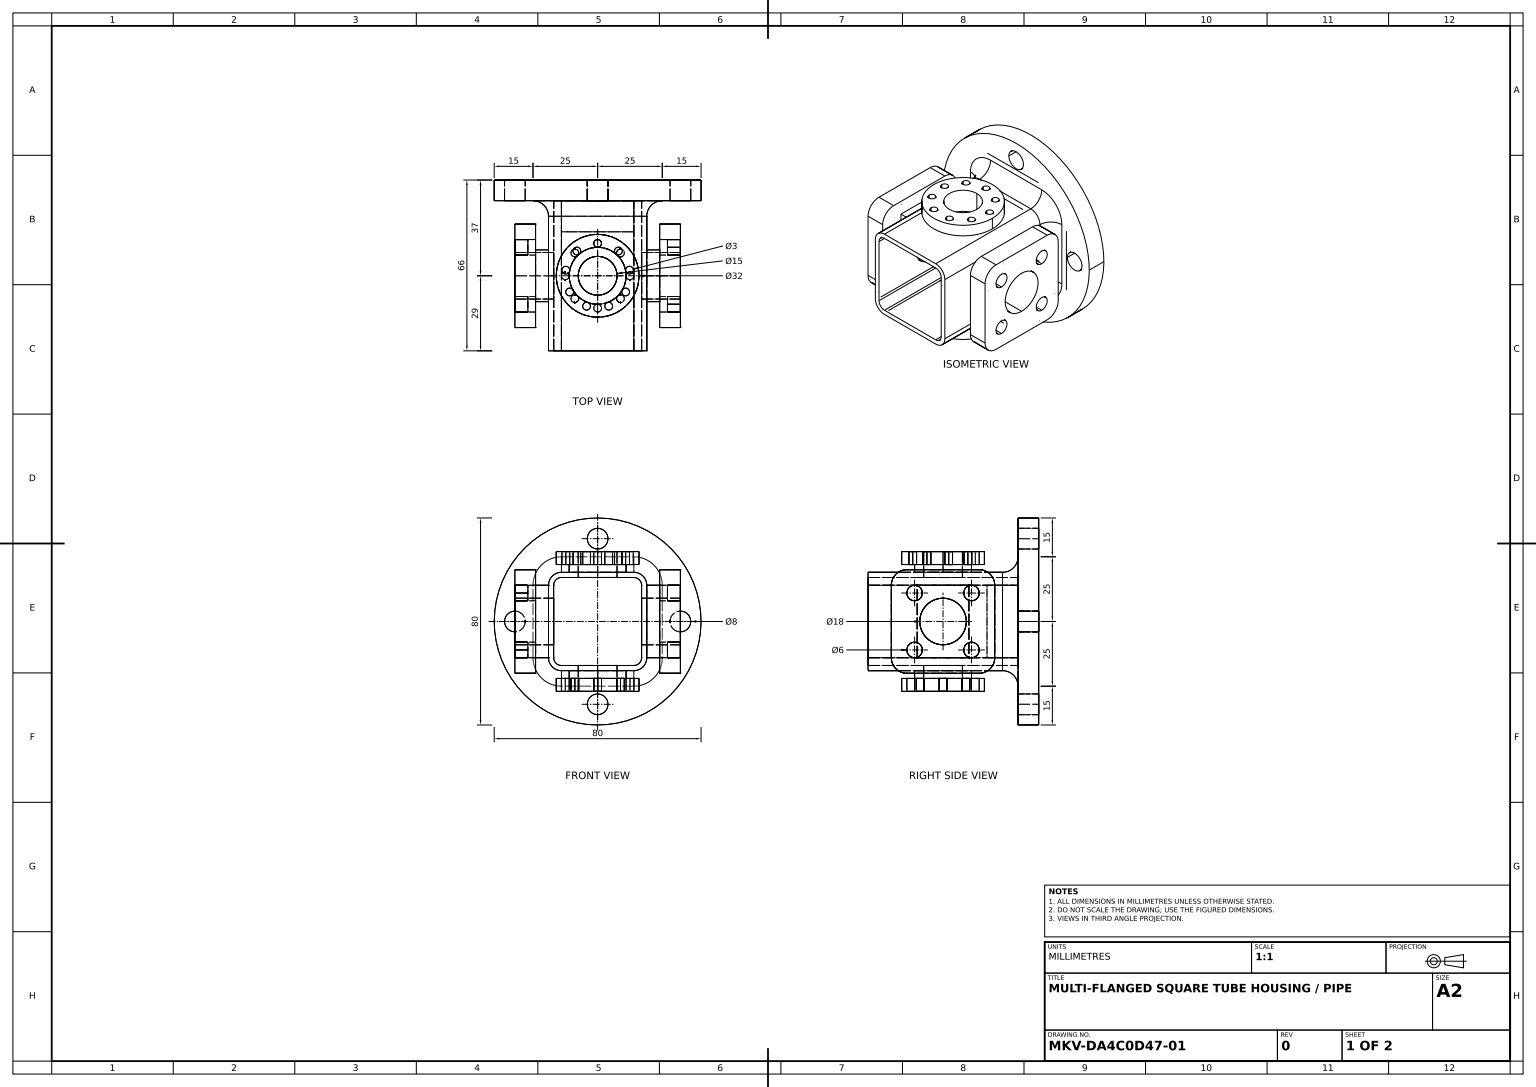
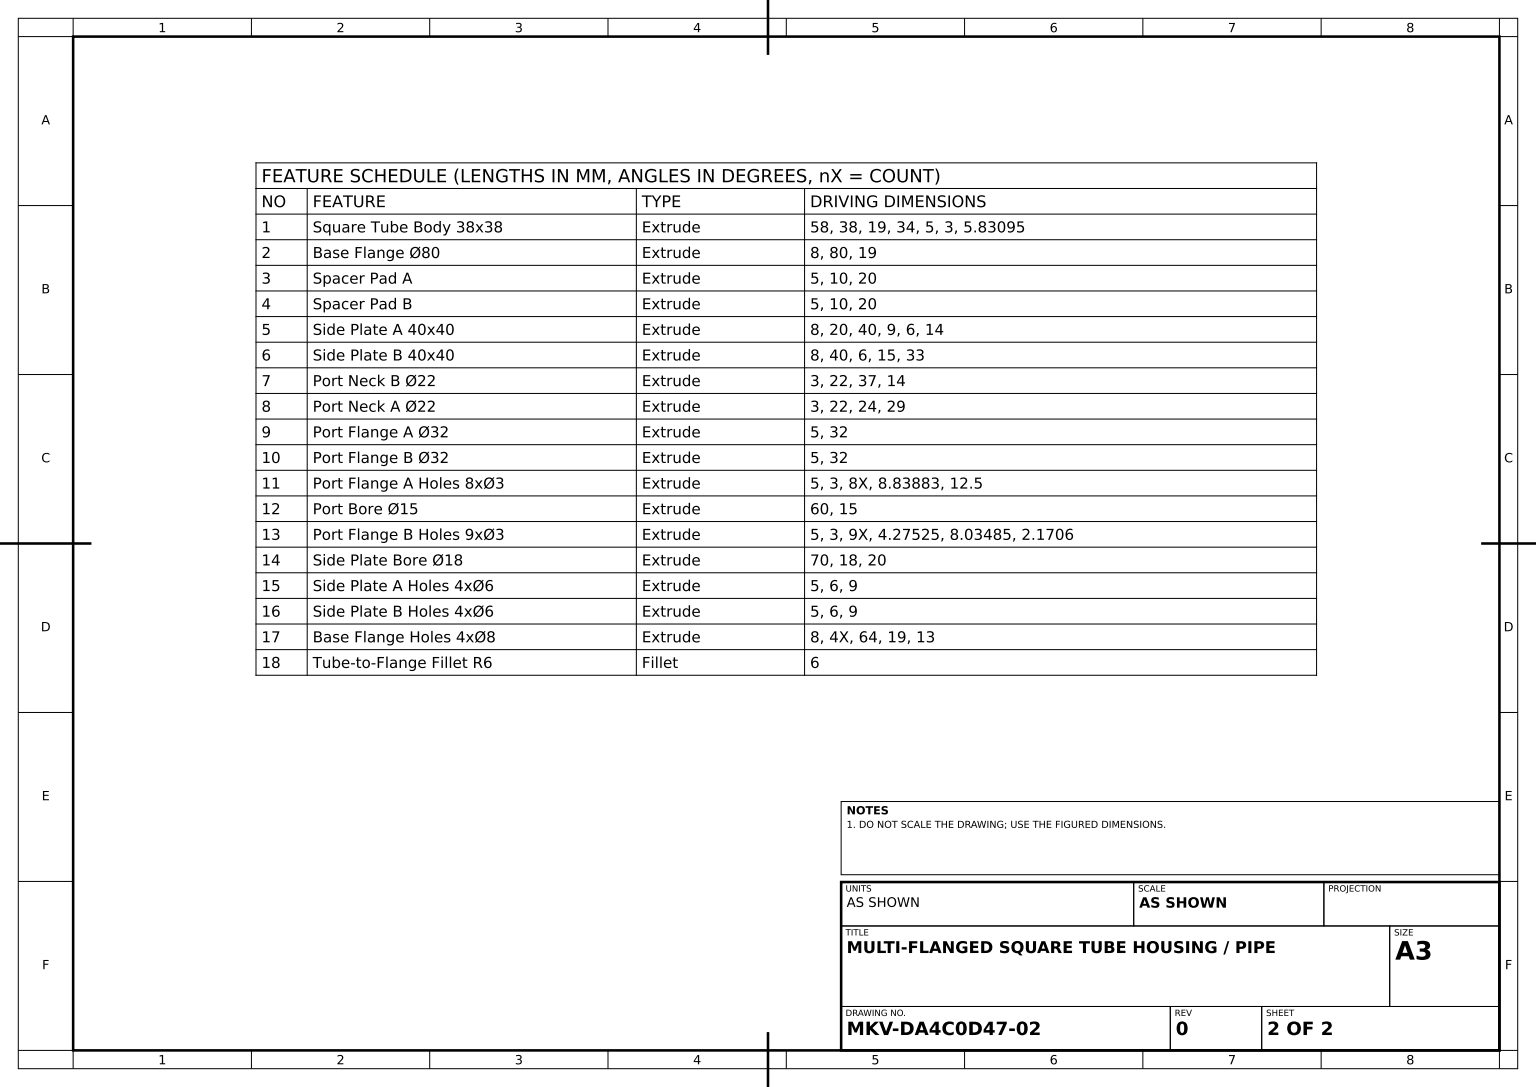
SolidWorks part; units mm, degrees
material "Plain Carbon Steel"
ref_plane "Front Plane" through (0, 0, 0) normal (0, 0, 1) x (1, 0, 0)
ref_plane "Top Plane" through (0, 0, 0) normal (0, 1, 0) x (1, 0, 0)
ref_plane "Right Plane" through (0, 0, 0) normal (1, 0, 0) x (0, 0, -1)
sketch "Square Tube Profile Sketch" plane through (0, 0, 0) normal (0, 0, 1) x (1, 0, 0)
  line L0 (5, 0) -> (33, 0)
  line L1 (38, -5) -> (38, -33)
  line L2 (33, -38) -> (5, -38)
  line L3 (0, -33) -> (0, -5)
  line L4 (5, -2) -> (33, -2)
  line L9 (36, -5) -> (36, -33)
  line L10 (33, -36) -> (5, -36)
  line L11 (2, -33) -> (2, -5)
  arc A0 (0, -5) -> (5, 0) centre (5, -5) cw
  arc A1 (38, -5) -> (33, 0) centre (33, -5) ccw
  arc A2 (33, -38) -> (38, -33) centre (33, -33) ccw
  arc A3 (5, -38) -> (0, -33) centre (5, -33) cw
  arc A4 (5, -36) -> (2, -33) centre (5, -33) cw
  arc A5 (33, -36) -> (36, -33) centre (33, -33) ccw
  arc A6 (36, -5) -> (33, -2) centre (33, -5) ccw
  arc A7 (5, -2) -> (2, -5) centre (5, -5) ccw
  point P5 (19, 0)
  point P8 (0, 0)
  point P19 (0, -38)
  point P28 (36, -19)
  dimension "D6" = 5
  dimension "D7" = 3
  dimension "D1" = 38
  dimension "D2" = 38
  dimension "D3" = 19
  dimension "D4" = 34
  dimension "D5" = 34
  dimension "D8" = 19
  dimension "D9" = 5.831
extrude "Square Tube Body 38x38" add sketch "Square Tube Profile Sketch" along normal blind 58
sketch "Base Flange Sketch" plane through (0, 0, 0) normal (0, 0, -1) x (-1, 0, 0)
  line L0 (0, -5) -> (0, -33) construction
  line L1 (-5, -38) -> (-33, -38) construction
  circle A0 centre (-19, -19) radius 40
  dimension "D1" = 80
  dimension "D2" = 19
  dimension "D3" = 19
extrude "Base Flange Ø80" add sketch "Base Flange Sketch" along normal blind 8
sketch "Spacer Pad A Sketch" plane through (38, 0, 0) normal (1, 0, 0) x (0, 0, -1)
  line L0 (-29, -5) -> (-19, -5)
  line L1 (-58, -5) -> (0, -5) construction
  line L2 (-19, -5) -> (-19, -33)
  line L3 (-58, -33) -> (0, -33) construction
  line L4 (-19, -33) -> (-39, -33)
  line L5 (-39, -33) -> (-39, -5)
  line L6 (-39, -5) -> (-19, -5)
  line M2 (0, -5) -> (-58, -5)
  line M4 (-58, -33) -> (0, -33)
  dimension "D1" = 10
  dimension "D2" = 20
extrude "Spacer Pad A" add sketch "Spacer Pad A Sketch" along normal blind 5 contours L5 L2 M4 M2
sketch "Spacer Pad B Sketch" plane through (0, 0, 0) normal (-1, 0, 0) x (0, 0, 1)
  line L0 (29, -5) -> (39, -5)
  line L1 (58, -5) -> (0, -5) construction
  line L2 (39, -5) -> (39, -33)
  line L3 (58, -33) -> (0, -33) construction
  line L4 (39, -33) -> (19, -33)
  line L5 (19, -33) -> (19, -5)
  line L6 (19, -5) -> (29, -5)
  dimension "D1" = 10
  dimension "D2" = 20
extrude "Spacer Pad B" add sketch "Spacer Pad B Sketch" along normal blind 5
sketch "Side Plate A Sketch" plane through (43, 0, 0) normal (1, 0, 0) x (0, 0, -1)
  line L0 (-58, -33) -> (-58, -5) construction
  line L2 (-9, -19) -> (-9, -5)
  line L3 (-15, 1) -> (-43, 1)
  line L4 (-49, -5) -> (-49, -33)
  line L5 (-43, -39) -> (-15, -39)
  line L6 (-9, -33) -> (-9, -19)
  line L7 (-39, -33) -> (-19, -33) construction
  arc A0 (-43, -39) -> (-49, -33) centre (-43, -33) cw
  arc A1 (-15, -39) -> (-9, -33) centre (-15, -33) ccw
  arc A2 (-9, -5) -> (-15, 1) centre (-15, -5) ccw
  arc A3 (-43, 1) -> (-49, -5) centre (-43, -5) ccw
  point P10 (-49, -39)
  point P15 (-9, 1)
  point P18 (-49, 1)
  dimension "D5" = 6
  dimension "D1" = 9
  dimension "D2" = 20
  dimension "D3" = 40
  dimension "D4" = 40
  dimension "D6" = 14
extrude "Side Plate A 40x40" add sketch "Side Plate A Sketch" along normal blind 8
sketch "Side Plate B Sketch" plane through (-5, 0, 0) normal (-1, 0, 0) x (0, 0, 1)
  line L0 (9, -5) -> (9, -33)
  line L3 (15, 1) -> (43, 1)
  line L4 (49, -5) -> (49, -33)
  line L5 (43, -39) -> (15, -39)
  arc A0 (15, -39) -> (9, -33) centre (15, -33) cw
  arc A1 (43, -39) -> (49, -33) centre (43, -33) ccw
  arc A2 (49, -5) -> (43, 1) centre (43, -5) ccw
  arc A3 (15, 1) -> (9, -5) centre (15, -5) ccw
  point P2 (9, -39)
  point P9 (49, -39)
  point P12 (49, 1)
  point P15 (9, 1)
  dimension "D1" = 6
  dimension "D2" = 15
  dimension "D3" = 40
  dimension "D4" = 40
  dimension "D5" = 40
  dimension "D6" = 33
extrude "Side Plate B 40x40" add sketch "Side Plate B Sketch" along normal blind 8
sketch "Port Neck B Sketch" plane through (0, 0, 0) normal (0, 1, 0) x (1, 0, 0)
  line L0 (59, 8) -> (-21, 8) construction
  line L1 (5, -58) -> (5, 0) construction
  circle A1 centre (19, -29) radius 11
  dimension "D1" = 37
  dimension "D2" = 22
  dimension "D3" = 14
extrude "Port Neck B Ø22" add sketch "Port Neck B Sketch" along normal blind 3
sketch "Port Neck A Sketch" plane through (0, -38, 0) normal (0, -1, 0) x (1, 0, 0)
  line L0 (43, 39) -> (43, 19) construction
  line L1 (5, 58) -> (33, 58) construction
  circle A0 centre (19, 29) radius 11
  dimension "D1" = 22
  dimension "D2" = 24
  dimension "D3" = 29
extrude "Port Neck A Ø22" add sketch "Port Neck A Sketch" along normal blind 3
sketch "Port Flange A Sketch" plane through (0, -41, 0) normal (0, -1, 0) x (1, 0, 0)
  circle A0 centre (19, 29) radius 16
  dimension "D1" = 32
extrude "Port Flange A Ø32" add sketch "Port Flange A Sketch" along normal blind 5
sketch "Port Flange B Sketch" plane through (0, 3, 0) normal (0, 1, 0) x (1, 0, 0)
  circle A0 centre (19, -29) radius 16
  dimension "D1" = 32
extrude "Port Flange B Ø32" add sketch "Port Flange B Sketch" along normal blind 5
sketch "Port Flange A Holes Sketch" plane through (0, -46, 0) normal (0, -1, 0) x (1, 0, 0)
  circle A1 centre (31.5, 29) radius 1.5
  circle A2 centre (27.8388, 20.1612) radius 1.5
  circle A3 centre (19, 16.5) radius 1.5
  circle A4 centre (10.1612, 20.1612) radius 1.5
  circle A5 centre (6.5, 29) radius 1.5
  circle A6 centre (10.1612, 37.8388) radius 1.5
  circle A7 centre (19, 41.5) radius 1.5
  circle A8 centre (27.8388, 37.8388) radius 1.5
  circle A9 centre (19, 29) radius 16 construction
  dimension "D1" = 8.8388
  dimension "D2" = 3
  dimension "D4" = 12.5
  dimension "D5" = 8.8388
  dimension "D3" = 8
extrude "Port Flange A Holes 8xØ3" cut sketch "Port Flange A Holes Sketch" against normal blind 5
sketch "Port Bore Sketch" plane through (0, -46, 0) normal (0, -1, 0) x (1, 0, 0)
  circle A0 centre (19, 29) radius 7.5
  dimension "D1" = 15
extrude "Port Bore Ø15" cut sketch "Port Bore Sketch" against normal blind 60
sketch "Port Flange B Holes Sketch" plane through (0, 8, 0) normal (0, 1, 0) x (1, 0, 0)
  circle A1 centre (19, -16.5) radius 1.5
  circle A2 centre (27.0348, -19.4244) radius 1.5
  circle A3 centre (31.3101, -26.8294) radius 1.5
  circle A4 centre (29.8253, -35.25) radius 1.5
  circle A5 centre (23.2753, -40.7462) radius 1.5
  circle A6 centre (14.7247, -40.7462) radius 1.5
  circle A7 centre (8.1747, -35.25) radius 1.5
  circle A8 centre (6.6899, -26.8294) radius 1.5
  circle A9 centre (10.9652, -19.4244) radius 1.5
  circle A10 centre (19, -29) radius 7.5 construction
  dimension "D1" = 4.2753
  dimension "D2" = 3
  dimension "D4" = 8.0348
  dimension "D5" = 2.1706
  dimension "D3" = 9
extrude "Port Flange B Holes 9xØ3" cut sketch "Port Flange B Holes Sketch" against normal blind 5
sketch "Side Plate Bore Sketch" plane through (51, 0, 0) normal (1, 0, 0) x (0, 0, -1)
  line L0 (-15, 1) -> (-43, 1) construction
  circle A0 centre (-29, -19) radius 9
  dimension "D1" = 18
  dimension "D2" = 20
  dimension "D3" = 20
extrude "Side Plate Bore Ø18" cut sketch "Side Plate Bore Sketch" against normal blind 70
sketch "Side Plate A Holes Sketch" plane through (51, 0, 0) normal (1, 0, 0) x (0, 0, -1)
  line L3 (-49, -5) -> (-49, -33) construction
  line L4 (-15, 1) -> (-43, 1) construction
  line L5 (-9, -33) -> (-9, -5) construction
  line L6 (-43, -39) -> (-15, -39) construction
  circle A1 centre (-18, -8) radius 3
  circle A2 centre (-40, -30) radius 3
  circle A3 centre (-18, -30) radius 3
  circle A4 centre (-40, -8) radius 3
  dimension "D2" = 6
  dimension "D3" = 6
  dimension "D4" = 6
  dimension "D5" = 6
  dimension "D6" = 9
  dimension "D7" = 9
  dimension "D8" = 9
  dimension "D9" = 9
  dimension "D10" = 9
  dimension "D11" = 9
  dimension "D12" = 9
  dimension "D13" = 9
extrude "Side Plate A Holes 4xØ6" cut sketch "Side Plate A Holes Sketch" against normal blind 5
sketch "Side Plate B Holes Sketch" plane through (-13, 0, 0) normal (-1, 0, 0) x (0, 0, 1)
  line L0 (9, -5) -> (9, -33) construction
  line L1 (43, 1) -> (15, 1) construction
  line L2 (15, -39) -> (43, -39) construction
  line L3 (49, -33) -> (49, -5) construction
  circle A0 centre (18, -8) radius 3
  circle A1 centre (40, -8) radius 3
  circle A2 centre (40, -30) radius 3
  circle A3 centre (18, -30) radius 3
  dimension "D1" = 6
  dimension "D2" = 6
  dimension "D3" = 6
  dimension "D4" = 6
  dimension "D5" = 9
  dimension "D6" = 9
  dimension "D7" = 9
  dimension "D8" = 9
  dimension "D9" = 9
  dimension "D10" = 9
  dimension "D11" = 9
  dimension "D12" = 9
extrude "Side Plate B Holes 4xØ6" cut sketch "Side Plate B Holes Sketch" against normal blind 5
sketch "Base Flange Holes Sketch" plane through (0, 0, -8) normal (0, 0, -1) x (-1, 0, 0)
  circle A1 centre (-19, 13) radius 4
  circle A2 centre (13, -19) radius 4
  circle A3 centre (-19, -51) radius 4
  circle A4 centre (-51, -19) radius 4
  dimension "D1" = 64
  dimension "D2" = 8
  dimension "D4" = 19
  dimension "D5" = 13
  dimension "D3" = 4
extrude "Base Flange Holes 4xØ8" cut sketch "Base Flange Holes Sketch" against normal blind 8
fillet "Tube-to-Flange Fillet R6" radius 6 8 edges at (1.4645, -36.5355, 0) (0, -19, 0) (1.4645, -1.4645, 0) (19, 0, 0) (36.5355, -1.4645, 0) (38, -19, 0) (36.5355, -36.5355, 0) (19, -38, 0)
